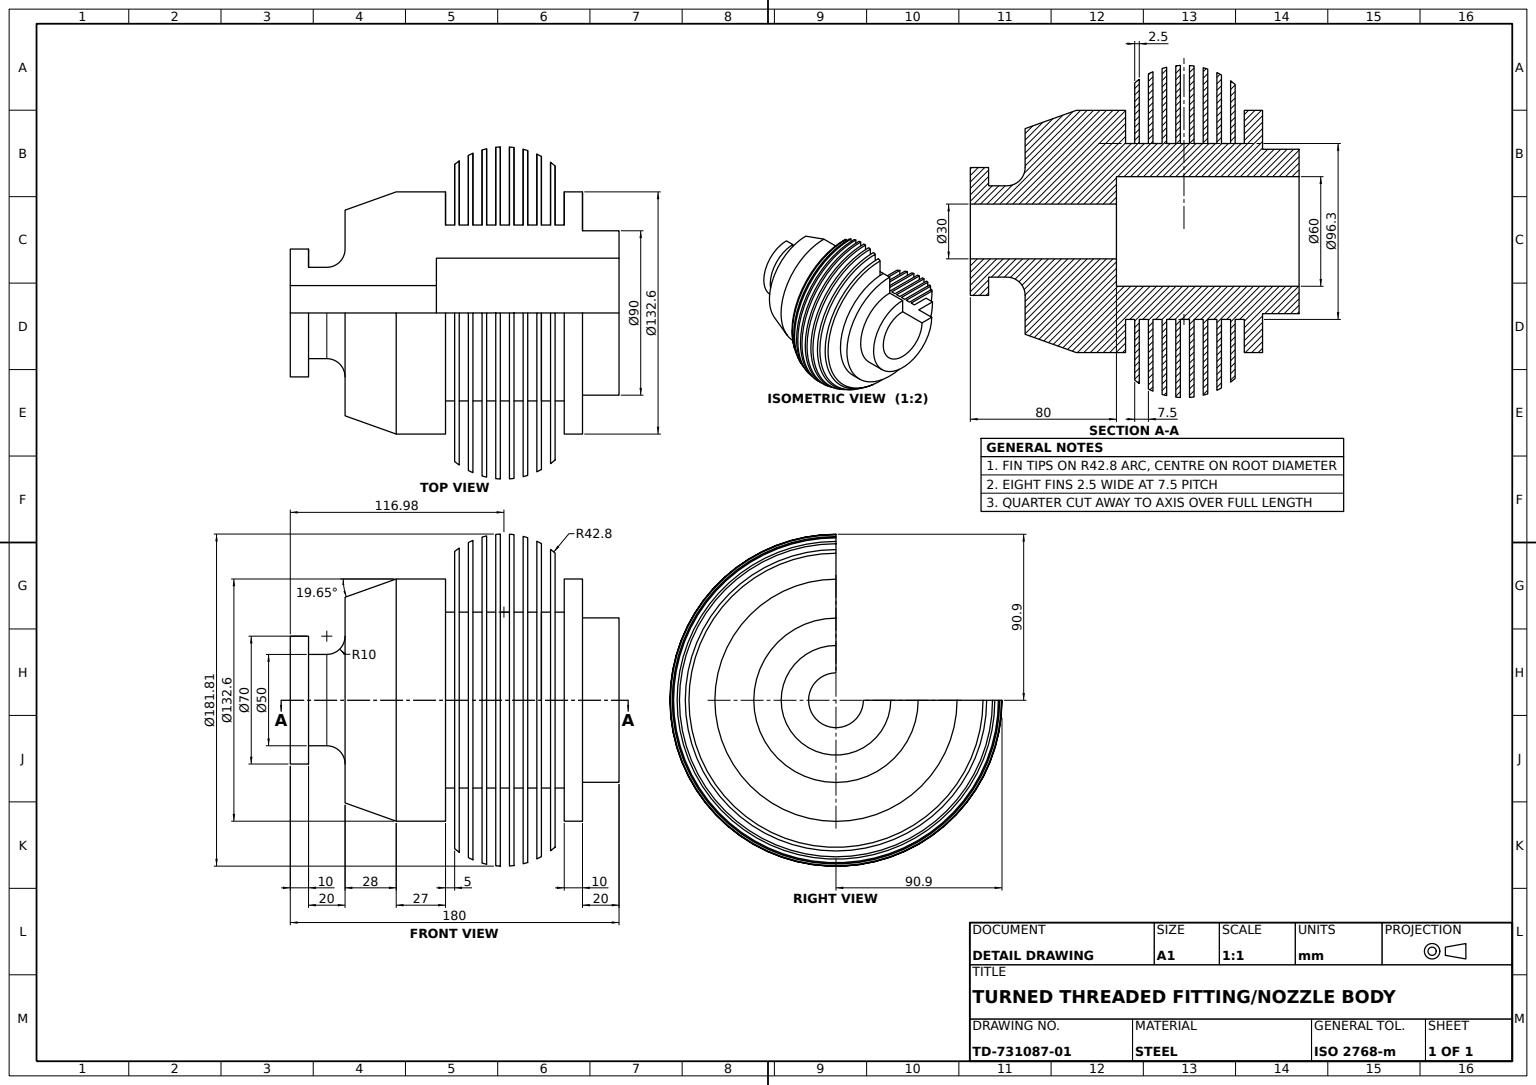
SolidWorks part; units mm, degrees
material "Plain Carbon Steel"
ref_plane "Front Plane" through (0, 0, 0) normal (0, 0, 1) x (1, 0, 0)
ref_plane "Top Plane" through (0, 0, 0) normal (0, 1, 0) x (1, 0, 0)
ref_plane "Right Plane" through (0, 0, 0) normal (1, 0, 0) x (0, 0, -1)
sketch "Shaft Profile Sketch" plane through (0, 0, 0) normal (0, 1, 0) x (1, 0, 0)
  line L3 (51.1564, 36.6745) -> (51.1564, 51.6745)
  line L15 (51.1564, 51.6745) -> (31.1564, 51.6745)
  line L16 (31.1564, 51.6745) -> (31.1564, 72.9745)
  line L17 (31.1564, 72.9745) -> (21.1564, 72.9745)
  line L18 (51.1564, 36.6745) -> (-48.8436, 36.6745)
  line L19 (-48.8436, 36.6745) -> (-48.8436, 21.6745)
  line L20 (-48.8436, 21.6745) -> (-128.8436, 21.6745)
  line L21 (-128.8436, 21.6745) -> (-128.8436, 41.6745)
  line L22 (-128.8436, 41.6745) -> (-118.8436, 41.6745)
  line L23 (-118.8436, 41.6745) -> (-118.8436, 31.6745)
  line L24 (-118.8436, 31.6745) -> (-108.8436, 31.6745)
  line L25 (-98.8436, 41.6745) -> (-98.8436, 62.9745)
  line L26 (-98.8436, 52.3245) -> (-93.9517, 52.3245)
  line L27 (-93.9517, 52.3245) -> (-101.8735, 52.3245)
  line L28 (-101.8735, 54.8245) -> (-93.9517, 54.8245)
  line L29 (-43.8436, 54.8245) -> (-38.8436, 54.8245)
  line L30 (21.1564, 72.9745) -> (21.1564, 54.8245)
  line L31 (16.1564, 75.2555) -> (16.1564, 54.8245)
  line L32 (16.1564, 75.2555) -> (16.1564, 87.1765)
  line L33 (13.6564, 75.2555) -> (13.6564, 54.8245)
  line L34 (13.6564, 75.2555) -> (13.6564, 89.1831)
  line L35 (8.6564, 75.2555) -> (8.6564, 54.8245)
  line L36 (8.6564, 75.2555) -> (8.6564, 92.3841)
  line L37 (6.1564, 75.2555) -> (6.1564, 54.8245)
  line L38 (6.1564, 75.2555) -> (6.1564, 93.6456)
  line L39 (1.1564, 75.2555) -> (1.1564, 95.5957)
  line L40 (1.1564, 75.2555) -> (1.1564, 54.8245)
  line L41 (-1.3436, 75.2555) -> (-1.3436, 54.8245)
  line L42 (-1.3436, 75.2555) -> (-1.3436, 96.3112)
  line L43 (-6.3436, 75.2555) -> (-6.3436, 97.2669)
  line L44 (-6.3436, 75.2555) -> (-6.3436, 54.8245)
  line L45 (-8.8436, 75.2555) -> (-8.8436, 54.8245)
  line L46 (-8.8436, 92.7206) -> (-8.8436, 97.5177)
  line L47 (-13.8436, 75.2555) -> (-13.8436, 97.5787)
  line L48 (-13.8436, 75.2555) -> (-13.8436, 54.8245)
  line L49 (-16.3436, 75.2555) -> (-16.3436, 54.8245)
  line L50 (-16.3436, 75.2555) -> (-16.3436, 97.3895)
  line L51 (-21.3436, 75.2555) -> (-21.3436, 54.8245)
  line L52 (-21.3436, 75.2555) -> (-21.3436, 96.5617)
  line L53 (-23.8436, 75.2555) -> (-23.8436, 95.914)
  line L54 (-23.8436, 75.2555) -> (-23.8436, 54.8245)
  line L55 (-28.8436, 75.2555) -> (-28.8436, 54.8245)
  line L56 (-28.8436, 75.2555) -> (-28.8436, 94.1126)
  line L57 (-31.3436, 75.2555) -> (-31.3436, 92.935)
  line L58 (-31.3436, 75.2555) -> (-31.3436, 54.8245)
  line L59 (-36.3436, 75.2555) -> (-36.3436, 54.8245)
  line L60 (-36.3436, 75.2555) -> (-36.3436, 89.9333)
  line L61 (-38.8436, 75.2555) -> (-38.8436, 88.0507)
  line L62 (-38.8436, 75.2555) -> (-38.8436, 54.8245)
  line L63 (-43.8436, 72.9745) -> (-43.8436, 54.8245)
  line L64 (-43.8436, 75.2555) -> (-43.8436, 48.0222) construction
  line L65 (-43.8436, 72.9745) -> (-70.8436, 72.9745)
  line L66 (-70.8436, 72.9745) -> (-98.8436, 62.9745)
  line L67 (-8.8436, 75.2555) -> (-8.8436, 138.0431) construction
  line L68 (-38.8436, 75.2555) -> (-38.8436, 138.0431) construction
  line L69 (-36.3436, 75.2555) -> (-36.3436, 138.0431) construction
  line L70 (-43.8436, 75.2555) -> (-43.8436, 138.0431) construction
  line L71 (-31.3436, 75.2555) -> (-31.3436, 138.0431) construction
  line L72 (-28.8436, 75.2555) -> (-28.8436, 138.0431) construction
  line L73 (-23.8436, 75.2555) -> (-23.8436, 138.0431) construction
  line L74 (-21.3436, 75.2555) -> (-21.3436, 138.0431) construction
  line L75 (-16.3436, 75.2555) -> (-16.3436, 138.0431) construction
  line L76 (-13.8436, 75.2555) -> (-13.8436, 138.0431) construction
  line L77 (-6.3436, 75.2555) -> (-6.3436, 138.0431) construction
  line L78 (-1.3436, 75.2555) -> (-1.3436, 138.0431) construction
  line L79 (1.1564, 75.2555) -> (1.1564, 138.0431) construction
  line L80 (6.1564, 75.2555) -> (6.1564, 138.0431) construction
  line L81 (8.6564, 75.2555) -> (8.6564, 138.0431) construction
  line L82 (13.6564, 75.2555) -> (13.6564, 138.0431) construction
  line L83 (16.1564, 75.2555) -> (16.1564, 138.0431) construction
  line L84 (-8.8436, 92.7206) -> (-8.8436, 75.2555)
  line L85 (-36.3436, 54.8245) -> (-31.3436, 54.8245)
  line L86 (21.1564, 75.2555) -> (21.1564, 48.0222) construction
  line L87 (16.1564, 75.2555) -> (16.1564, 48.0222) construction
  line L88 (13.6564, 75.2555) -> (13.6564, 48.0222) construction
  line L89 (8.6564, 75.2555) -> (8.6564, 48.0222) construction
  line L90 (6.1564, 75.2555) -> (6.1564, 48.0222) construction
  line L91 (1.1564, 75.2555) -> (1.1564, 48.0222) construction
  line L92 (-1.3436, 75.2555) -> (-1.3436, 48.0222) construction
  line L93 (-6.3436, 75.2555) -> (-6.3436, 48.0222) construction
  line L94 (-8.8436, 75.2555) -> (-8.8436, 48.0222) construction
  line L95 (-13.8436, 75.2555) -> (-13.8436, 48.0222) construction
  line L96 (-16.3436, 75.2555) -> (-16.3436, 48.0222) construction
  line L97 (-21.3436, 75.2555) -> (-21.3436, 48.0222) construction
  line L98 (-23.8436, 75.2555) -> (-23.8436, 48.0222) construction
  line L99 (-28.8436, 75.2555) -> (-28.8436, 48.0222) construction
  line L100 (-31.3436, 75.2555) -> (-31.3436, 48.0222) construction
  line L101 (-36.3436, 75.2555) -> (-36.3436, 48.0222) construction
  line L102 (-38.8436, 75.2555) -> (-38.8436, 48.0222) construction
  line L103 (-28.8436, 54.8245) -> (-23.8436, 54.8245)
  line L104 (-21.3436, 54.8245) -> (-16.3436, 54.8245)
  line L105 (-13.8436, 54.8245) -> (-8.8436, 54.8245)
  line L106 (-6.3436, 54.8245) -> (-1.3436, 54.8245)
  line L107 (1.1564, 54.8245) -> (6.1564, 54.8245)
  line L108 (8.6564, 54.8245) -> (13.6564, 54.8245)
  line L109 (16.1564, 54.8245) -> (21.1564, 54.8245)
  line L110 (-11.3436, 54.8245) -> (-11.3436, 36.6745)
  line L111 (-18.8436, 54.8245) -> (-18.8436, 36.6745)
  line L112 (-3.8436, 54.8245) -> (-3.8436, 36.6745)
  line L113 (-149.6058, 6.6745) -> (74.5845, 6.6745) construction
  arc A0 (-98.8436, 41.6745) -> (-108.8436, 31.6745) centre (-108.8436, 41.6745) cw
  arc A2 (-36.3436, 89.9333) -> (-38.8436, 88.0507) centre (-11.8648, 54.8245) ccw
  arc A3 (-28.8436, 94.1126) -> (-31.3436, 92.935) centre (-11.8648, 54.8245) ccw
  arc A4 (-21.3436, 96.5617) -> (-23.8436, 95.914) centre (-11.8648, 54.8245) ccw
  arc A5 (-13.8436, 97.5787) -> (-16.3436, 97.3895) centre (-11.8648, 54.8245) ccw
  arc A6 (-6.3436, 97.2669) -> (-8.8436, 97.5177) centre (-11.8648, 54.8245) ccw
  arc A7 (1.1564, 95.5957) -> (-1.3436, 96.3112) centre (-11.8648, 54.8245) ccw
  arc A8 (8.6564, 92.3841) -> (6.1564, 93.6456) centre (-11.8648, 54.8245) ccw
  arc A9 (16.1564, 87.1765) -> (13.6564, 89.1831) centre (-11.8648, 54.8245) ccw
  point P16 (-98.8436, 31.6745)
  dimension "D11" = 10
  dimension "D31" = 7.5
  dimension "D44" = 42.8
  dimension "D1" = 15
  dimension "D2" = 20
  dimension "D3" = 21.3
  dimension "D4" = 10
  dimension "D5" = 100
  dimension "D6" = 15
  dimension "D7" = 80
  dimension "D8" = 20
  dimension "D9" = 10
  dimension "D10" = 20
  dimension "D12" = 21.3
  dimension "D13" = 2.5
  dimension "D32" = 7.5
  dimension "D33" = 15
  dimension "D34" = 6.6745
  dimension "D35" = 128.8436
  dimension "D36" = 20.7622
  dimension "D37" = 23.4281
  dimension "D38" = 4.8919
  dimension "D39" = 7.9218
  dimension "D40" = 27
  dimension "D41" = 18.15
  dimension "D42" = 20.431
  dimension "D43" = 17.4651
  dimension "D45" = 0.5211
  dimension "D14" = 5
  dimension "D15" = 2.5
  dimension "D16" = 5
  dimension "D17" = 2.5
  dimension "D18" = 5
  dimension "D19" = 2.5
  dimension "D20" = 5
  dimension "D21" = 2.5
  dimension "D22" = 5
  dimension "D23" = 2.5
  dimension "D24" = 5
  dimension "D25" = 2.5
  dimension "D26" = 5
  dimension "D27" = 2.5
  dimension "D28" = 5
  dimension "D29" = 2.5
  dimension "D30" = 5
revolve "Revolved Shaft Body" add sketch "Shaft Profile Sketch" angle 360 about L113
sketch "Slot Cut Sketch" plane through (51.1564, 0, 0) normal (1, 0, 0) x (0, 0, -1)
  line L0 (6.6745, 0) -> (6.6745, 99.7163)
  line L1 (6.6745, 99.7163) -> (6.6745, 0)
  line L2 (105.779, 0) -> (105.779, 99.7163)
  line L3 (105.779, 99.7163) -> (6.6745, 99.7163)
  line L4 (6.6745, 0) -> (105.779, 0)
  circle A0 centre (6.6745, 0) radius 45 construction
  circle M1 centre (6.6745, 0) radius 45
  circle M2 centre (6.6745, 0) radius 30
  dimension "D1" = 99.1045
  dimension "D2" = 99.7163
extrude "Slot Cut" cut sketch "Slot Cut Sketch" against normal blind 267 and the other way blind 81 contours L4 L2 L3 L0 M1 | L4 L0 M2 M1 | L0 L4 M2
